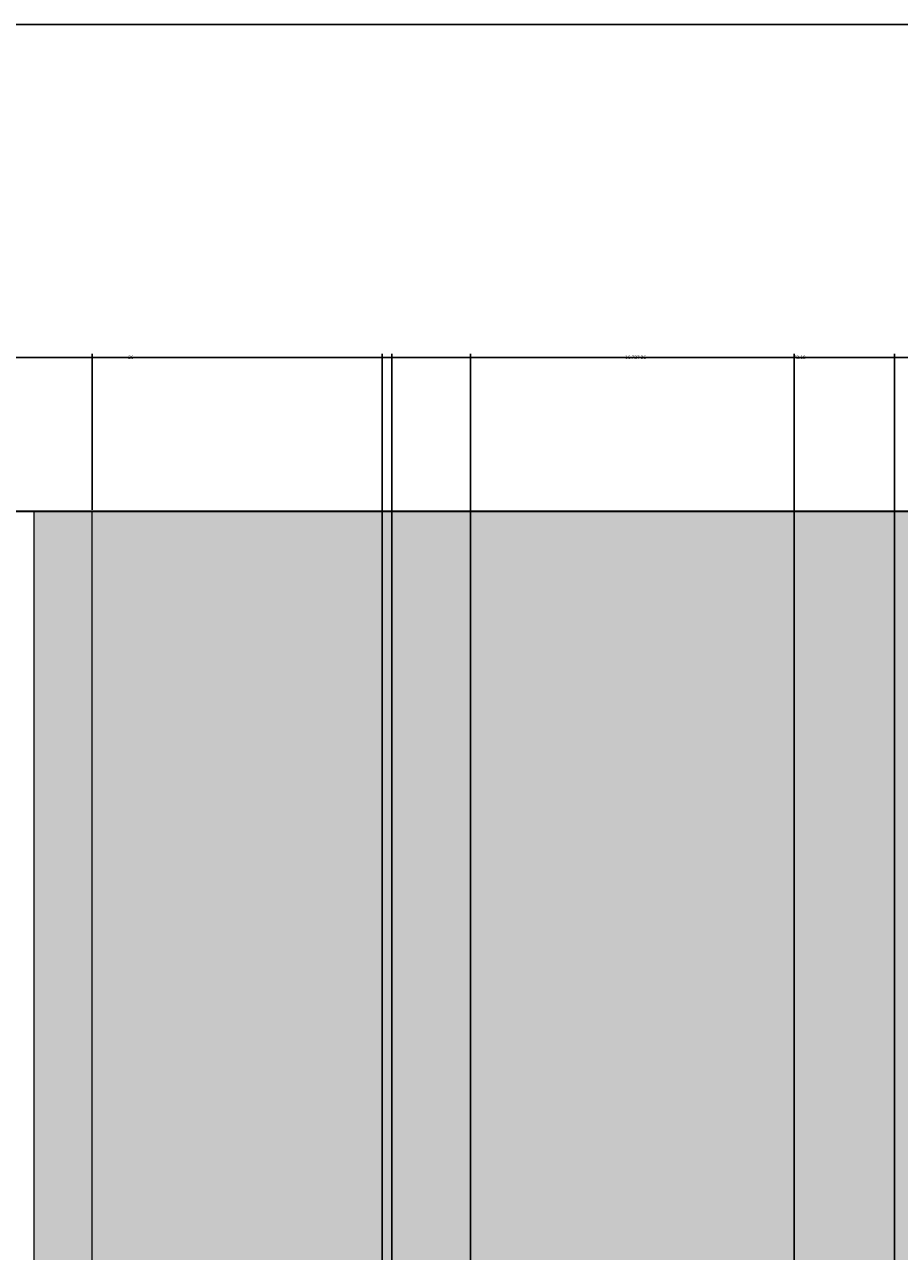
# Model space of a CAD drawing. Units: inches. Extents: x 4508 to 4723, y 847 to 1020.
# Tile 17 of 32: x 4585 to 4631, y 956 to 1020. Entities that reach past the tile are written whole.
import ezdxf

# ---------------------------------------------------------------- set-up
doc = ezdxf.new("R2010")
doc.units = ezdxf.units.IN
for name, color, linetype, lineweight in [('A-ANNO-DIMS', 2, 'Continuous', 18), ('A-ANNO-TTLB', 7, 'Continuous', 25), ('A-WALL', 7, 'Continuous', 35), ('A-WALL-FINS', 30, 'Continuous', 18), ('A-WALL-PATT', 254, 'Continuous', 13)]:
    doc.layers.add(name, color=color, linetype=linetype, lineweight=lineweight)
doc.styles.get("Standard").update_dxf_attribs({"font": 'arial.ttf'})
doc.dimstyles.get("Standard").update_dxf_attribs({"dimtxt": 0.18, "dimasz": 0.18, "dimexe": 0.18, "dimexo": 0.0625, "dimgap": 0.09, "dimtad": 0, "dimtih": 1, "dimtoh": 1, "dimdec": 4, "dimzin": 0, "dimdsep": 46, "dimtxsty": 'Standard', "dimcen": 0.09, "dimadec": 0, "dimazin": 0, "dimtfac": 1, "dimtdec": 4, "dimtofl": 0, "dimtmove": 0, "dimatfit": 3, "dimfxl": 1, "dimtolj": 1, "dimtzin": 0, "dimarcsym": 0})

# ---------------------------------------------------------------- blocks, each defined once
blk = doc.blocks.new('*D7')
at = {"layer": 'A-ANNO-DIMS', "color": 0, "lineweight": -2, "transparency": 16777216}
for p, q in [((4588.994, 994.809), (4588.994, 1002.877)), ((4662.171, 957.665), (4662.171, 1002.877)), ((4589.174, 1002.697), (4625.189, 1002.697)), ((4661.991, 1002.697), (4625.975, 1002.697))]:
    blk.add_line(p, q, dxfattribs=at)
at = {"layer": 'A-ANNO-DIMS', "color": 0, "lineweight": 9, "transparency": 16777216}
for points in [[(4589.174, 1002.727), (4589.174, 1002.667), (4588.994, 1002.697)], [(4661.991, 1002.727), (4661.991, 1002.667), (4662.171, 1002.697)]]:
    blk.add_solid(points, dxfattribs=at)
at = {"layer": 'Defpoints', "color": 0, "lineweight": 9, "transparency": 16777216}
for p in [(4662.171, 1002.697), (4588.994, 994.747), (4662.171, 957.602)]:
    blk.add_point(p, dxfattribs=at)
at = {"layer": 'A-ANNO-DIMS', "color": 0, "transparency": 16777216, "insert": (4625.582, 1002.697), "char_height": 0.18, "attachment_point": 5}
blk.add_mtext('\\A1;73.18', dxfattribs=at)
blk = doc.blocks.new('*D29')
at = {"layer": 'A-ANNO-DIMS', "color": 0, "lineweight": -2, "transparency": 16777216}
for p, q in [((4577.994, 903.809), (4577.994, 1002.877)), ((4603.994, 903.809), (4603.994, 1002.877)), ((4578.174, 1002.697), (4590.773, 1002.697)), ((4603.814, 1002.697), (4591.214, 1002.697))]:
    blk.add_line(p, q, dxfattribs=at)
at = {"layer": 'A-ANNO-DIMS', "color": 0, "lineweight": 9, "transparency": 16777216}
for points in [[(4578.174, 1002.727), (4578.174, 1002.667), (4577.994, 1002.697)], [(4603.814, 1002.727), (4603.814, 1002.667), (4603.994, 1002.697)]]:
    blk.add_solid(points, dxfattribs=at)
at = {"layer": 'Defpoints', "color": 0, "lineweight": 9, "transparency": 16777216}
for p in [(4603.994, 1002.697), (4577.994, 903.747), (4603.994, 903.747)]:
    blk.add_point(p, dxfattribs=at)
at = {"layer": 'A-ANNO-DIMS', "color": 0, "transparency": 16777216, "insert": (4590.994, 1002.697), "char_height": 0.18, "attachment_point": 5}
blk.add_mtext('\\A1;26', dxfattribs=at)
blk = doc.blocks.new('*D30')
at = {"layer": 'A-ANNO-DIMS', "color": 0, "lineweight": -2, "transparency": 16777216}
for p, q in [((4604.494, 903.809), (4604.494, 1002.877)), ((4630.494, 903.809), (4630.494, 1002.877)), ((4604.674, 1002.697), (4617.273, 1002.697)), ((4630.314, 1002.697), (4617.714, 1002.697))]:
    blk.add_line(p, q, dxfattribs=at)
at = {"layer": 'A-ANNO-DIMS', "color": 0, "lineweight": 9, "transparency": 16777216}
for points in [[(4604.674, 1002.727), (4604.674, 1002.667), (4604.494, 1002.697)], [(4630.314, 1002.727), (4630.314, 1002.667), (4630.494, 1002.697)]]:
    blk.add_solid(points, dxfattribs=at)
at = {"layer": 'Defpoints', "color": 0, "lineweight": 9, "transparency": 16777216}
for p in [(4630.494, 1002.697), (4604.494, 903.747), (4630.494, 903.747)]:
    blk.add_point(p, dxfattribs=at)
at = {"layer": 'A-ANNO-DIMS', "color": 0, "transparency": 16777216, "insert": (4617.494, 1002.697), "char_height": 0.18, "attachment_point": 5}
blk.add_mtext('\\A1;26', dxfattribs=at)
blk = doc.blocks.new('*D34')
at = {"layer": 'A-ANNO-DIMS', "color": 0, "lineweight": -2, "transparency": 16777216}
for p, q in [((4608.562, 892.49), (4608.562, 1002.877)), ((4625.298, 892.49), (4625.298, 1002.877)), ((4608.742, 1002.697), (4616.475, 1002.697)), ((4625.118, 1002.697), (4617.385, 1002.697))]:
    blk.add_line(p, q, dxfattribs=at)
at = {"layer": 'A-ANNO-DIMS', "color": 0, "lineweight": 9, "transparency": 16777216}
for points in [[(4608.742, 1002.727), (4608.742, 1002.667), (4608.562, 1002.697)], [(4625.118, 1002.727), (4625.118, 1002.667), (4625.298, 1002.697)]]:
    blk.add_solid(points, dxfattribs=at)
at = {"layer": 'Defpoints', "color": 0, "lineweight": 9, "transparency": 16777216}
for p in [(4625.298, 1002.697), (4608.562, 892.428), (4625.298, 892.428)]:
    blk.add_point(p, dxfattribs=at)
at = {"layer": 'A-ANNO-DIMS', "color": 0, "transparency": 16777216, "insert": (4616.93, 1002.697), "char_height": 0.18, "attachment_point": 5}
blk.add_mtext('\\A1;16.737', dxfattribs=at)

msp = doc.modelspace()

# ---------------------------------------------------------------- hatches: boundary and pattern name
at = {"layer": 'A-WALL-PATT', "transparency": 33554508}
h = msp.add_hatch(color=256, dxfattribs=at)
h.dxf.hatch_style = 1
h.paths.add_polyline_path([(4661.6706, 954.043, -0.3739004), (4658.5765, 957.6021, -1), (4665.7646, 957.6021, -0.3739004), (4662.6706, 954.043), (4662.6706, 944.4021, -0.2114781), (4670.3062, 945.0869), (4670.3062, 968.0592, -0.4632086), (4663.3246, 973.9783, -0.4632086), (4670.3062, 979.8975), (4670.3062, 994.7469), (4588.9938, 994.7469), (4588.9938, 904.7469), (4657.9938, 904.7469), (4657.9938, 886.7469), (4549.9938, 886.7469), (4549.9938, 878.7469), (4693.9938, 878.7469), (4693.9938, 994.7469), (4671.8062, 994.7469), (4671.8062, 979.4411, -0.2941682), (4675.3246, 973.9783, -0.2941682), (4671.8062, 968.5156), (4671.8062, 944.4278, -0.2741114), (4676.7298, 936.1217, -0.2741114), (4671.8062, 927.8155), (4671.8062, 907.6998, -0.3779645), (4677.0562, 901.7469, -0.3779645), (4671.8062, 895.7939), (4671.8062, 883.7469), (4670.3062, 883.7469), (4670.3062, 895.7939, -0.3779645), (4665.0562, 901.7469, -0.3779645), (4670.3062, 907.6998), (4670.3062, 927.1564, -0.2114781), (4662.6706, 927.8412), (4662.6706, 918.2003, -0.3739004), (4665.7646, 914.6412, -1), (4658.5765, 914.6412, -0.3739004), (4661.6706, 918.2003), (4661.6706, 928.4807, -0.2391825), (4657.7936, 936.1217, -0.2391825), (4661.6706, 943.7626)])
at = {"layer": 'A-WALL-PATT', "transparency": 33554681}
h = msp.add_hatch(color=256, dxfattribs=at)
h.dxf.hatch_style = 1
h.paths.add_polyline_path([(4588.9938, 994.7469), (4585.9938, 994.7469), (4585.9938, 904.7469), (4588.9938, 904.7469)])

# ---------------------------------------------------------------- linework, layer by layer
at = {"layer": 'A-ANNO-TTLB'}
msp.add_lwpolyline([(4508.3867, 1019.9118), (4722.9774, 1019.9118), (4722.9774, 846.9535), (4508.3867, 846.9535)], close=True, dxfattribs=at)
at = {"layer": 'A-WALL'}
msp.add_line((4540.9938, 994.7469), (4693.9938, 994.7469), dxfattribs=at)
at = {"layer": 'A-WALL-FINS'}
for p, q in [((4585.9938, 904.7469), (4585.9938, 994.7469)), ((4588.9938, 904.7469), (4588.9938, 994.7469))]:
    msp.add_line(p, q, dxfattribs=at)

# ---------------------------------------------------------------- dimensions: what is measured, and where the dimension line sits
at = {"layer": 'A-ANNO-DIMS'}
for base, p1, p2, override, picture, middle in [((4603.9938, 1002.6969), (4577.9938, 903.7469), (4603.9938, 903.7469), {"dimdec": 0, "dimlfac": 1, "dimrnd": 0, "dimzin": 0, "dimdsep": 46, "dimlunit": 2}, '*D29', (4590.9938, 1002.6969)), ((4662.1706, 1002.6969), (4588.9938, 994.7469), (4662.1706, 957.6021), {"dimdec": 2, "dimlfac": 1, "dimrnd": 0, "dimzin": 0, "dimdsep": 46, "dimlunit": 2}, '*D7', (4625.5822, 1002.6969)), ((4630.4938, 1002.6969), (4604.4938, 903.7469), (4630.4938, 903.7469), {"dimdec": 0, "dimlfac": 1, "dimrnd": 0, "dimzin": 0, "dimdsep": 46, "dimlunit": 2}, '*D30', (4617.4938, 1002.6969)), ((4625.2983, 1002.6969), (4608.5617, 892.4277), (4625.2983, 892.4277), {"dimdec": 3, "dimlfac": 1, "dimrnd": 0, "dimzin": 0, "dimdsep": 46, "dimlunit": 2}, '*D34', (4616.93, 1002.6969))]:
    dim = msp.add_linear_dim(base=base, p1=p1, p2=p2, dimstyle='Standard', override=override, dxfattribs=at)
    dim.commit()
    dim.dimension.update_dxf_attribs({"geometry": picture, "text_midpoint": middle})

doc.saveas('drawing.dxf')
